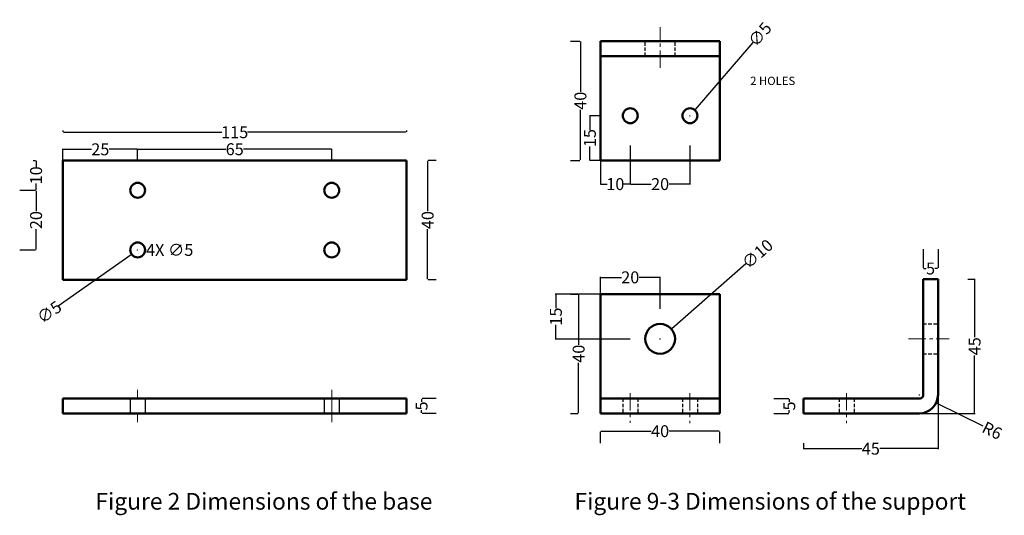
# Model space of a CAD drawing. Units: millimetres. Extents: x 1183 to 1513, y 471 to 941.
# Tile 3 of 3: x 1183 to 1513, y 775 to 941. Entities that reach past the tile are written whole.
import ezdxf

# ---------------------------------------------------------------- set-up
doc = ezdxf.new("R2010")
doc.units = ezdxf.units.MM
doc.header["$LTSCALE"] = 1.4
doc.header["$MEASUREMENT"] = 0
doc.linetypes.add('CENTER', pattern=[50.8, 31.75, -6.35, 6.35, -6.35])
doc.linetypes.add('HIDDEN', pattern=[9.525, 6.35, -3.175])
for name, color, linetype, lineweight in [('M-CNTR', 1, 'CENTER', 18), ('M-DIMS', 2, 'Continuous', 25), ('M-HIDN', 4, 'HIDDEN', 25), ('M-OUTL', 7, 'Continuous', 50), ('M-TEXT', 3, 'Continuous', 25)]:
    doc.layers.add(name, color=color, linetype=linetype, lineweight=lineweight)
doc.styles.get("Standard").update_dxf_attribs({"font": 'arial.ttf'})
doc.dimstyles.get("Standard").update_dxf_attribs({"dimtxt": 4, "dimasz": 0.18, "dimexe": 0.18, "dimexo": 10, "dimgap": 0.09, "dimtad": 0, "dimdec": 0, "dimzin": 0, "dimdsep": 46, "dimtxsty": 'Standard', "dimcen": 0.09, "dimadec": 0, "dimazin": 0, "dimtfac": 1, "dimtdec": 0, "dimtofl": 0, "dimtmove": 0, "dimatfit": 3, "dimfxl": 1, "dimtolj": 1, "dimtzin": 0, "dimarcsym": 0})

# ---------------------------------------------------------------- blocks, each defined once
blk = doc.blocks.new('*D1')
at = {"layer": 'Defpoints', "color": 0, "lineweight": 140, "ltscale": 0.13, "transparency": 16777216}
for p in [(1312.98, 903.47), (1197.98, 894.01), (1312.98, 894.01)]:
    blk.add_point(p, dxfattribs=at)
at = {"layer": 'M-DIMS', "color": 0, "lineweight": -2, "ltscale": 0.13, "transparency": 16777216}
for p, q in [((1197.98, 904.01), (1197.98, 903.65)), ((1198.16, 903.47), (1251.15, 903.47)), ((1312.8, 903.47), (1259.82, 903.47)), ((1312.98, 904.01), (1312.98, 903.65))]:
    blk.add_line(p, q, dxfattribs=at)
at = {"layer": 'M-DIMS', "color": 0, "lineweight": 140, "ltscale": 0.13, "transparency": 16777216}
for points in [[(1198.16, 903.5), (1198.16, 903.44), (1197.98, 903.47)], [(1312.8, 903.5), (1312.8, 903.44), (1312.98, 903.47)]]:
    blk.add_solid(points, dxfattribs=at)
at = {"layer": 'M-DIMS', "color": 0, "ltscale": 0.13, "transparency": 16777216, "insert": (1255.48, 903.47), "char_height": 4, "attachment_point": 5}
blk.add_mtext('\\A1;115', dxfattribs=at)
blk = doc.blocks.new('*D2')
at = {"layer": 'Defpoints', "color": 0, "lineweight": 140, "ltscale": 0.13, "transparency": 16777216}
for p in [(1287.98, 897.77), (1222.98, 884.01), (1287.98, 884.01)]:
    blk.add_point(p, dxfattribs=at)
at = {"layer": 'M-DIMS', "color": 0, "lineweight": -2, "ltscale": 0.13, "transparency": 16777216}
for p, q in [((1222.98, 894.01), (1222.98, 897.95)), ((1223.16, 897.77), (1252.5, 897.77)), ((1287.8, 897.77), (1258.46, 897.77)), ((1287.98, 894.01), (1287.98, 897.95))]:
    blk.add_line(p, q, dxfattribs=at)
at = {"layer": 'M-DIMS', "color": 0, "lineweight": 140, "ltscale": 0.13, "transparency": 16777216}
for points in [[(1223.16, 897.8), (1223.16, 897.74), (1222.98, 897.77)], [(1287.8, 897.8), (1287.8, 897.74), (1287.98, 897.77)]]:
    blk.add_solid(points, dxfattribs=at)
at = {"layer": 'M-DIMS', "color": 0, "ltscale": 0.13, "transparency": 16777216, "insert": (1255.48, 897.77), "char_height": 4, "attachment_point": 5}
blk.add_mtext('\\A1;65', dxfattribs=at)
blk = doc.blocks.new('*D3')
at = {"layer": 'Defpoints', "color": 0, "lineweight": 140, "ltscale": 0.13, "transparency": 16777216}
for p in [(1197.98, 897.74), (1197.98, 884.01), (1222.98, 884.01)]:
    blk.add_point(p, dxfattribs=at)
at = {"layer": 'M-DIMS', "color": 0, "lineweight": -2, "ltscale": 0.13, "transparency": 16777216}
for p, q in [((1197.98, 894.01), (1197.98, 897.92)), ((1198.16, 897.74), (1207.48, 897.74)), ((1222.8, 897.74), (1213.49, 897.74)), ((1222.98, 894.01), (1222.98, 897.92))]:
    blk.add_line(p, q, dxfattribs=at)
at = {"layer": 'M-DIMS', "color": 0, "lineweight": 140, "ltscale": 0.13, "transparency": 16777216}
for points in [[(1198.16, 897.77), (1198.16, 897.71), (1197.98, 897.74)], [(1222.8, 897.77), (1222.8, 897.71), (1222.98, 897.74)]]:
    blk.add_solid(points, dxfattribs=at)
at = {"layer": 'M-DIMS', "color": 0, "ltscale": 0.13, "transparency": 16777216, "insert": (1210.48, 897.74), "char_height": 4, "attachment_point": 5}
blk.add_mtext('\\A1;25', dxfattribs=at)
blk = doc.blocks.new('*D4')
at = {"layer": 'Defpoints', "color": 0, "lineweight": 140, "ltscale": 0.13, "transparency": 16777216}
for p in [(1188.97, 884.01), (1193.48, 884.01), (1193.48, 864.01)]:
    blk.add_point(p, dxfattribs=at)
at = {"layer": 'M-DIMS', "color": 0, "lineweight": -2, "ltscale": 0.13, "transparency": 16777216}
for p, q in [((1183.48, 884.01), (1188.79, 884.01)), ((1188.97, 883.83), (1188.97, 876.99)), ((1188.97, 864.19), (1188.97, 871.02)), ((1183.48, 864.01), (1188.79, 864.01))]:
    blk.add_line(p, q, dxfattribs=at)
at = {"layer": 'M-DIMS', "color": 0, "lineweight": 140, "ltscale": 0.13, "transparency": 16777216}
for points in [[(1188.94, 883.83), (1189, 883.83), (1188.97, 884.01)], [(1188.94, 864.19), (1189, 864.19), (1188.97, 864.01)]]:
    blk.add_solid(points, dxfattribs=at)
at = {"layer": 'M-DIMS', "color": 0, "ltscale": 0.13, "transparency": 16777216, "insert": (1188.97, 874.01), "char_height": 4, "attachment_point": 5, "rotation": 90}
blk.add_mtext('\\A1;20', dxfattribs=at)
blk = doc.blocks.new('*D5')
at = {"layer": 'Defpoints', "color": 0, "lineweight": 140, "ltscale": 0.13, "transparency": 16777216}
for p in [(1197.98, 894.01), (1188.97, 884.01), (1197.98, 884.01)]:
    blk.add_point(p, dxfattribs=at)
at = {"layer": 'M-DIMS', "color": 0, "lineweight": -2, "ltscale": 0.13, "transparency": 16777216}
for p, q in [((1187.98, 894.01), (1188.79, 894.01)), ((1188.97, 893.83), (1188.97, 891.77)), ((1187.98, 884.01), (1188.79, 884.01)), ((1188.97, 884.19), (1188.97, 886.25))]:
    blk.add_line(p, q, dxfattribs=at)
at = {"layer": 'M-DIMS', "color": 0, "lineweight": 140, "ltscale": 0.13, "transparency": 16777216}
for points in [[(1188.94, 893.83), (1189, 893.83), (1188.97, 894.01)], [(1188.94, 884.19), (1189, 884.19), (1188.97, 884.01)]]:
    blk.add_solid(points, dxfattribs=at)
at = {"layer": 'M-DIMS', "color": 0, "ltscale": 0.13, "transparency": 16777216, "insert": (1188.97, 889.01), "char_height": 4, "attachment_point": 5, "rotation": 90}
blk.add_mtext('\\A1;10', dxfattribs=at)
blk = doc.blocks.new('*D6')
at = {"layer": 'Defpoints', "color": 0, "lineweight": 140, "ltscale": 0.13, "transparency": 16777216}
for p in [(1225.03, 865.44), (1220.94, 862.57)]:
    blk.add_point(p, dxfattribs=at)
at = {"layer": 'M-DIMS', "color": 0, "lineweight": -2, "ltscale": 0.13, "transparency": 16777216}
for p, q in [((1222.89, 864.01), (1223.07, 864.01)), ((1222.98, 863.92), (1222.98, 864.1)), ((1196.32, 845.25), (1220.79, 862.46))]:
    blk.add_line(p, q, dxfattribs=at)
at = {"layer": 'M-DIMS', "color": 0, "lineweight": 140, "ltscale": 0.13, "transparency": 16777216}
blk.add_solid([(1220.77, 862.49), (1220.81, 862.44), (1220.94, 862.57)], dxfattribs=at)
at = {"layer": 'M-DIMS', "color": 0, "ltscale": 0.13, "transparency": 16777216, "insert": (1193.38, 843.18), "char_height": 4, "attachment_point": 5, "rotation": 35.1278}
blk.add_mtext('\\A1;∅5', dxfattribs=at)
blk = doc.blocks.new('*D7')
at = {"layer": 'Defpoints', "color": 0, "lineweight": 140, "ltscale": 0.13, "transparency": 16777216}
for p in [(1312.98, 894.01), (1312.98, 854.01), (1320.09, 854.01)]:
    blk.add_point(p, dxfattribs=at)
at = {"layer": 'M-DIMS', "color": 0, "lineweight": -2, "ltscale": 0.13, "transparency": 16777216}
for p, q in [((1320.09, 893.83), (1320.09, 877.03)), ((1322.98, 894.01), (1320.27, 894.01)), ((1320.09, 854.19), (1320.09, 870.98)), ((1322.98, 854.01), (1320.27, 854.01))]:
    blk.add_line(p, q, dxfattribs=at)
at = {"layer": 'M-DIMS', "color": 0, "lineweight": 140, "ltscale": 0.13, "transparency": 16777216}
for points in [[(1320.06, 893.83), (1320.12, 893.83), (1320.09, 894.01)], [(1320.06, 854.19), (1320.12, 854.19), (1320.09, 854.01)]]:
    blk.add_solid(points, dxfattribs=at)
at = {"layer": 'M-DIMS', "color": 0, "ltscale": 0.13, "transparency": 16777216, "insert": (1320.09, 874.01), "char_height": 4, "attachment_point": 5, "rotation": 90}
blk.add_mtext('\\A1;40', dxfattribs=at)
blk = doc.blocks.new('*D8')
at = {"layer": 'Defpoints', "color": 0, "lineweight": 140, "ltscale": 0.13, "transparency": 16777216}
for p in [(1371.24, 934.01), (1377.94, 934.01), (1377.94, 894.01)]:
    blk.add_point(p, dxfattribs=at)
at = {"layer": 'M-DIMS', "color": 0, "lineweight": -2, "ltscale": 0.13, "transparency": 16777216}
for p, q in [((1367.94, 934.01), (1371.06, 934.01)), ((1371.24, 933.83), (1371.24, 917.03)), ((1371.24, 894.19), (1371.24, 910.98)), ((1367.94, 894.01), (1371.06, 894.01))]:
    blk.add_line(p, q, dxfattribs=at)
at = {"layer": 'M-DIMS', "color": 0, "lineweight": 140, "ltscale": 0.13, "transparency": 16777216}
for points in [[(1371.21, 933.83), (1371.27, 933.83), (1371.24, 934.01)], [(1371.21, 894.19), (1371.27, 894.19), (1371.24, 894.01)]]:
    blk.add_solid(points, dxfattribs=at)
at = {"layer": 'M-DIMS', "color": 0, "ltscale": 0.13, "transparency": 16777216, "insert": (1371.24, 914.01), "char_height": 4, "attachment_point": 5, "rotation": 90}
blk.add_mtext('\\A1;40', dxfattribs=at)
blk = doc.blocks.new('*D9')
at = {"layer": 'Defpoints', "color": 0, "lineweight": 140, "ltscale": 0.13, "transparency": 16777216}
for p in [(1377.94, 909.01), (1387.94, 909.01), (1377.94, 886.08)]:
    blk.add_point(p, dxfattribs=at)
at = {"layer": 'M-DIMS', "color": 0, "lineweight": -2, "ltscale": 0.13, "transparency": 16777216}
for p, q in [((1377.94, 899.01), (1377.94, 885.9)), ((1387.94, 899.01), (1387.94, 885.9)), ((1378.12, 886.08), (1380.18, 886.08)), ((1387.76, 886.08), (1385.7, 886.08))]:
    blk.add_line(p, q, dxfattribs=at)
at = {"layer": 'M-DIMS', "color": 0, "lineweight": 140, "ltscale": 0.13, "transparency": 16777216}
for points in [[(1378.12, 886.11), (1378.12, 886.05), (1377.94, 886.08)], [(1387.76, 886.11), (1387.76, 886.05), (1387.94, 886.08)]]:
    blk.add_solid(points, dxfattribs=at)
at = {"layer": 'M-DIMS', "color": 0, "ltscale": 0.13, "transparency": 16777216, "insert": (1382.94, 886.08), "char_height": 4, "attachment_point": 5}
blk.add_mtext('\\A1;10', dxfattribs=at)
blk = doc.blocks.new('*D10')
at = {"layer": 'Defpoints', "color": 0, "lineweight": 140, "ltscale": 0.13, "transparency": 16777216}
for p in [(1387.94, 909.01), (1407.94, 909.01), (1407.94, 886.08)]:
    blk.add_point(p, dxfattribs=at)
at = {"layer": 'M-DIMS', "color": 0, "lineweight": -2, "ltscale": 0.13, "transparency": 16777216}
for p, q in [((1387.94, 899.01), (1387.94, 885.9)), ((1407.94, 899.01), (1407.94, 885.9)), ((1388.12, 886.08), (1394.96, 886.08)), ((1407.76, 886.08), (1400.92, 886.08))]:
    blk.add_line(p, q, dxfattribs=at)
at = {"layer": 'M-DIMS', "color": 0, "lineweight": 140, "ltscale": 0.13, "transparency": 16777216}
for points in [[(1388.12, 886.11), (1388.12, 886.05), (1387.94, 886.08)], [(1407.76, 886.11), (1407.76, 886.05), (1407.94, 886.08)]]:
    blk.add_solid(points, dxfattribs=at)
at = {"layer": 'M-DIMS', "color": 0, "ltscale": 0.13, "transparency": 16777216, "insert": (1397.94, 886.08), "char_height": 4, "attachment_point": 5}
blk.add_mtext('\\A1;20', dxfattribs=at)
blk = doc.blocks.new('*D11')
at = {"layer": 'Defpoints', "color": 0, "lineweight": 140, "ltscale": 0.13, "transparency": 16777216}
for p in [(1374.42, 909.01), (1387.94, 909.01), (1387.94, 894.01)]:
    blk.add_point(p, dxfattribs=at)
at = {"layer": 'M-DIMS', "color": 0, "lineweight": -2, "ltscale": 0.13, "transparency": 16777216}
for p, q in [((1377.94, 909.01), (1374.24, 909.01)), ((1374.42, 908.83), (1374.42, 904.29)), ((1374.42, 894.19), (1374.42, 898.72)), ((1377.94, 894.01), (1374.24, 894.01))]:
    blk.add_line(p, q, dxfattribs=at)
at = {"layer": 'M-DIMS', "color": 0, "lineweight": 140, "ltscale": 0.13, "transparency": 16777216}
for points in [[(1374.39, 908.83), (1374.45, 908.83), (1374.42, 909.01)], [(1374.39, 894.19), (1374.45, 894.19), (1374.42, 894.01)]]:
    blk.add_solid(points, dxfattribs=at)
at = {"layer": 'M-DIMS', "color": 0, "ltscale": 0.13, "transparency": 16777216, "insert": (1374.42, 901.51), "char_height": 4, "attachment_point": 5, "rotation": 90}
blk.add_mtext('\\A1;15', dxfattribs=at)
blk = doc.blocks.new('*D12')
at = {"layer": 'Defpoints', "color": 0, "lineweight": 140, "ltscale": 0.13, "transparency": 16777216}
for p in [(1409.57, 910.9), (1406.31, 907.11)]:
    blk.add_point(p, dxfattribs=at)
at = {"layer": 'M-DIMS', "color": 0, "lineweight": -2, "ltscale": 0.13, "transparency": 16777216}
for p, q in [((1429.01, 933.53), (1409.68, 911.04)), ((1407.85, 909.01), (1408.03, 909.01)), ((1407.94, 908.92), (1407.94, 909.1))]:
    blk.add_line(p, q, dxfattribs=at)
at = {"layer": 'M-DIMS', "color": 0, "lineweight": 140, "ltscale": 0.13, "transparency": 16777216}
blk.add_solid([(1409.66, 911.06), (1409.71, 911.02), (1409.57, 910.9)], dxfattribs=at)
at = {"layer": 'M-DIMS', "color": 0, "ltscale": 0.13, "transparency": 16777216, "insert": (1431.35, 936.26), "char_height": 4, "attachment_point": 5, "rotation": 49.3316}
blk.add_mtext('\\A1;∅5', dxfattribs=at)
blk = doc.blocks.new('*D13')
at = {"layer": 'Defpoints', "color": 0, "lineweight": 140, "ltscale": 0.13, "transparency": 16777216}
for p in [(1312.98, 814.23), (1318.05, 814.23), (1312.98, 809.23)]:
    blk.add_point(p, dxfattribs=at)
at = {"layer": 'M-DIMS', "color": 0, "lineweight": -2, "ltscale": 0.13, "transparency": 16777216}
for p, q in [((1318.05, 814.05), (1318.05, 813.14)), ((1322.98, 814.23), (1318.23, 814.23)), ((1318.05, 809.41), (1318.05, 810.31)), ((1322.98, 809.23), (1318.23, 809.23))]:
    blk.add_line(p, q, dxfattribs=at)
at = {"layer": 'M-DIMS', "color": 0, "lineweight": 140, "ltscale": 0.13, "transparency": 16777216}
for points in [[(1318.02, 814.05), (1318.08, 814.05), (1318.05, 814.23)], [(1318.02, 809.41), (1318.08, 809.41), (1318.05, 809.23)]]:
    blk.add_solid(points, dxfattribs=at)
at = {"layer": 'M-DIMS', "color": 0, "ltscale": 0.13, "transparency": 16777216, "insert": (1318.05, 811.73), "char_height": 4, "attachment_point": 5, "rotation": 90}
blk.add_mtext('\\A1;5', dxfattribs=at)
blk = doc.blocks.new('*D14')
at = {"layer": 'Defpoints', "color": 0, "lineweight": 140, "ltscale": 0.13, "transparency": 16777216}
for p in [(1377.94, 854.83), (1377.94, 834.23), (1397.94, 834.23)]:
    blk.add_point(p, dxfattribs=at)
at = {"layer": 'M-DIMS', "color": 0, "lineweight": -2, "ltscale": 0.13, "transparency": 16777216}
for p, q in [((1377.94, 844.23), (1377.94, 855.01)), ((1378.12, 854.83), (1384.96, 854.83)), ((1397.76, 854.83), (1390.92, 854.83)), ((1397.94, 844.23), (1397.94, 855.01))]:
    blk.add_line(p, q, dxfattribs=at)
at = {"layer": 'M-DIMS', "color": 0, "lineweight": 140, "ltscale": 0.13, "transparency": 16777216}
for points in [[(1378.12, 854.86), (1378.12, 854.8), (1377.94, 854.83)], [(1397.76, 854.86), (1397.76, 854.8), (1397.94, 854.83)]]:
    blk.add_solid(points, dxfattribs=at)
at = {"layer": 'M-DIMS', "color": 0, "ltscale": 0.13, "transparency": 16777216, "insert": (1387.94, 854.83), "char_height": 4, "attachment_point": 5}
blk.add_mtext('\\A1;20', dxfattribs=at)
blk = doc.blocks.new('*D15')
at = {"layer": 'Defpoints', "color": 0, "lineweight": 140, "ltscale": 0.13, "transparency": 16777216}
for p in [(1370.65, 849.23), (1377.94, 849.23), (1377.94, 809.23)]:
    blk.add_point(p, dxfattribs=at)
at = {"layer": 'M-DIMS', "color": 0, "lineweight": -2, "ltscale": 0.13, "transparency": 16777216}
for p, q in [((1367.94, 849.23), (1370.47, 849.23)), ((1370.65, 849.05), (1370.65, 832.25)), ((1370.65, 809.41), (1370.65, 826.2)), ((1367.94, 809.23), (1370.47, 809.23))]:
    blk.add_line(p, q, dxfattribs=at)
at = {"layer": 'M-DIMS', "color": 0, "lineweight": 140, "ltscale": 0.13, "transparency": 16777216}
for points in [[(1370.62, 849.05), (1370.68, 849.05), (1370.65, 849.23)], [(1370.62, 809.41), (1370.68, 809.41), (1370.65, 809.23)]]:
    blk.add_solid(points, dxfattribs=at)
at = {"layer": 'M-DIMS', "color": 0, "ltscale": 0.13, "transparency": 16777216, "insert": (1370.65, 829.23), "char_height": 4, "attachment_point": 5, "rotation": 90}
blk.add_mtext('\\A1;40', dxfattribs=at)
blk = doc.blocks.new('*D16')
at = {"layer": 'Defpoints', "color": 0, "lineweight": 140, "ltscale": 0.13, "transparency": 16777216}
for p in [(1377.94, 809.23), (1417.94, 809.23), (1417.94, 803.28)]:
    blk.add_point(p, dxfattribs=at)
at = {"layer": 'M-DIMS', "color": 0, "lineweight": -2, "ltscale": 0.13, "transparency": 16777216}
for p, q in [((1377.94, 799.23), (1377.94, 803.1)), ((1378.12, 803.28), (1394.91, 803.28)), ((1417.76, 803.28), (1400.97, 803.28)), ((1417.94, 799.23), (1417.94, 803.1))]:
    blk.add_line(p, q, dxfattribs=at)
at = {"layer": 'M-DIMS', "color": 0, "lineweight": 140, "ltscale": 0.13, "transparency": 16777216}
for points in [[(1378.12, 803.31), (1378.12, 803.25), (1377.94, 803.28)], [(1417.76, 803.31), (1417.76, 803.25), (1417.94, 803.28)]]:
    blk.add_solid(points, dxfattribs=at)
at = {"layer": 'M-DIMS', "color": 0, "ltscale": 0.13, "transparency": 16777216, "insert": (1397.94, 803.28), "char_height": 4, "attachment_point": 5}
blk.add_mtext('\\A1;40', dxfattribs=at)
blk = doc.blocks.new('*D17')
at = {"layer": 'Defpoints', "color": 0, "lineweight": 140, "ltscale": 0.13, "transparency": 16777216}
for p in [(1401.7, 837.52), (1394.17, 830.94)]:
    blk.add_point(p, dxfattribs=at)
at = {"layer": 'M-DIMS', "color": 0, "lineweight": -2, "ltscale": 0.13, "transparency": 16777216}
for p, q in [((1426.66, 859.33), (1401.84, 837.63)), ((1397.85, 834.23), (1398.03, 834.23)), ((1397.94, 834.14), (1397.94, 834.32))]:
    blk.add_line(p, q, dxfattribs=at)
at = {"layer": 'M-DIMS', "color": 0, "lineweight": 140, "ltscale": 0.13, "transparency": 16777216}
blk.add_solid([(1401.82, 837.66), (1401.86, 837.61), (1401.7, 837.52)], dxfattribs=at)
at = {"layer": 'M-DIMS', "color": 0, "ltscale": 0.13, "transparency": 16777216, "insert": (1430.52, 862.7), "char_height": 4, "attachment_point": 5, "rotation": 41.1476}
blk.add_mtext('\\A1;∅10', dxfattribs=at)
blk = doc.blocks.new('*D18')
at = {"layer": 'Defpoints', "color": 0, "lineweight": 140, "ltscale": 0.13, "transparency": 16777216}
for p in [(1484.75, 815.48), (1490.36, 812.72)]:
    blk.add_point(p, dxfattribs=at)
at = {"layer": 'M-DIMS', "color": 0, "lineweight": -2, "ltscale": 0.13, "transparency": 16777216}
for p, q in [((1484.66, 815.48), (1484.84, 815.48)), ((1484.75, 815.39), (1484.75, 815.57)), ((1506.15, 804.95), (1490.52, 812.64))]:
    blk.add_line(p, q, dxfattribs=at)
at = {"layer": 'M-DIMS', "color": 0, "lineweight": 140, "ltscale": 0.13, "transparency": 16777216}
blk.add_solid([(1490.53, 812.66), (1490.5, 812.61), (1490.36, 812.72)], dxfattribs=at)
at = {"layer": 'M-DIMS', "color": 0, "ltscale": 0.13, "transparency": 16777216, "insert": (1509.13, 803.48), "char_height": 4, "attachment_point": 5, "rotation": 333.8095}
blk.add_mtext('\\A1;R6', dxfattribs=at)
blk = doc.blocks.new('*D19')
at = {"layer": 'Defpoints', "color": 0, "lineweight": 140, "ltscale": 0.13, "transparency": 16777216}
for p in [(1363.03, 849.23), (1397.94, 849.23), (1397.94, 834.14)]:
    blk.add_point(p, dxfattribs=at)
at = {"layer": 'M-DIMS', "color": 0, "lineweight": -2, "ltscale": 0.13, "transparency": 16777216}
for p, q in [((1387.94, 849.23), (1362.85, 849.23)), ((1363.03, 849.05), (1363.03, 844.46)), ((1363.03, 834.32), (1363.03, 838.9)), ((1387.94, 834.14), (1362.85, 834.14))]:
    blk.add_line(p, q, dxfattribs=at)
at = {"layer": 'M-DIMS', "color": 0, "lineweight": 140, "ltscale": 0.13, "transparency": 16777216}
for points in [[(1363, 849.05), (1363.06, 849.05), (1363.03, 849.23)], [(1363, 834.32), (1363.06, 834.32), (1363.03, 834.14)]]:
    blk.add_solid(points, dxfattribs=at)
at = {"layer": 'M-DIMS', "color": 0, "ltscale": 0.13, "transparency": 16777216, "insert": (1363.03, 841.68), "char_height": 4, "attachment_point": 5, "rotation": 90}
blk.add_mtext('\\A1;15', dxfattribs=at)
blk = doc.blocks.new('*D20')
at = {"layer": 'Defpoints', "color": 0, "lineweight": 140, "ltscale": 0.13, "transparency": 16777216}
for p in [(1491, 857.79), (1486, 854.23), (1491, 854.23)]:
    blk.add_point(p, dxfattribs=at)
at = {"layer": 'M-DIMS', "color": 0, "lineweight": -2, "ltscale": 0.13, "transparency": 16777216}
for p, q in [((1486, 864.23), (1486, 857.97)), ((1491, 864.23), (1491, 857.97)), ((1486.18, 857.79), (1487.08, 857.79)), ((1490.82, 857.79), (1489.91, 857.79))]:
    blk.add_line(p, q, dxfattribs=at)
at = {"layer": 'M-DIMS', "color": 0, "lineweight": 140, "ltscale": 0.13, "transparency": 16777216}
for points in [[(1486.18, 857.82), (1486.18, 857.76), (1486, 857.79)], [(1490.82, 857.82), (1490.82, 857.76), (1491, 857.79)]]:
    blk.add_solid(points, dxfattribs=at)
at = {"layer": 'M-DIMS', "color": 0, "ltscale": 0.13, "transparency": 16777216, "insert": (1488.5, 857.79), "char_height": 4, "attachment_point": 5}
blk.add_mtext('\\A1;5', dxfattribs=at)
blk = doc.blocks.new('*D21')
at = {"layer": 'Defpoints', "color": 0, "lineweight": 140, "ltscale": 0.13, "transparency": 16777216}
for p in [(1441.17, 814.23), (1446, 814.23), (1446, 809.23)]:
    blk.add_point(p, dxfattribs=at)
at = {"layer": 'M-DIMS', "color": 0, "lineweight": -2, "ltscale": 0.13, "transparency": 16777216}
for p, q in [((1436, 814.23), (1440.99, 814.23)), ((1441.17, 814.05), (1441.17, 813.14)), ((1436, 809.23), (1440.99, 809.23)), ((1441.17, 809.41), (1441.17, 810.31))]:
    blk.add_line(p, q, dxfattribs=at)
at = {"layer": 'M-DIMS', "color": 0, "lineweight": 140, "ltscale": 0.13, "transparency": 16777216}
for points in [[(1441.14, 814.05), (1441.2, 814.05), (1441.17, 814.23)], [(1441.14, 809.41), (1441.2, 809.41), (1441.17, 809.23)]]:
    blk.add_solid(points, dxfattribs=at)
at = {"layer": 'M-DIMS', "color": 0, "ltscale": 0.13, "transparency": 16777216, "insert": (1441.17, 811.73), "char_height": 4, "attachment_point": 5, "rotation": 90}
blk.add_mtext('\\A1;5', dxfattribs=at)
blk = doc.blocks.new('*D46')
at = {"layer": 'Defpoints', "color": 0, "lineweight": 140, "ltscale": 1.4, "transparency": 16777216}
for p in [(1491, 854.23), (1446, 809.23), (1491, 797.42)]:
    blk.add_point(p, dxfattribs=at)
at = {"layer": 'M-DIMS', "color": 0, "lineweight": -2, "ltscale": 1.4, "transparency": 16777216}
for p, q in [((1491, 844.23), (1491, 797.24)), ((1446, 799.23), (1446, 797.24)), ((1446.18, 797.42), (1465.45, 797.42)), ((1490.82, 797.42), (1471.55, 797.42))]:
    blk.add_line(p, q, dxfattribs=at)
at = {"layer": 'M-DIMS', "color": 0, "lineweight": 140, "ltscale": 1.4, "transparency": 16777216}
for points in [[(1446.18, 797.45), (1446.18, 797.39), (1446, 797.42)], [(1490.82, 797.45), (1490.82, 797.39), (1491, 797.42)]]:
    blk.add_solid(points, dxfattribs=at)
at = {"layer": 'M-DIMS', "color": 0, "ltscale": 1.4, "transparency": 16777216, "insert": (1468.5, 797.42), "char_height": 4, "attachment_point": 5}
blk.add_mtext('\\A1;45', dxfattribs=at)
blk = doc.blocks.new('*D47')
at = {"layer": 'Defpoints', "color": 0, "lineweight": 140, "ltscale": 1.4, "transparency": 16777216}
for p in [(1491, 854.23), (1503.24, 854.23), (1446, 809.23)]:
    blk.add_point(p, dxfattribs=at)
at = {"layer": 'M-DIMS', "color": 0, "lineweight": -2, "ltscale": 1.4, "transparency": 16777216}
for p, q in [((1501, 854.23), (1503.42, 854.23)), ((1503.24, 854.05), (1503.24, 834.78)), ((1503.24, 809.41), (1503.24, 828.68)), ((1456, 809.23), (1503.42, 809.23))]:
    blk.add_line(p, q, dxfattribs=at)
at = {"layer": 'M-DIMS', "color": 0, "lineweight": 140, "ltscale": 1.4, "transparency": 16777216}
for points in [[(1503.21, 854.05), (1503.27, 854.05), (1503.24, 854.23)], [(1503.21, 809.41), (1503.27, 809.41), (1503.24, 809.23)]]:
    blk.add_solid(points, dxfattribs=at)
at = {"layer": 'M-DIMS', "color": 0, "ltscale": 1.4, "transparency": 16777216, "insert": (1503.24, 831.73), "char_height": 4, "attachment_point": 5, "rotation": 90}
blk.add_mtext('\\A1;45', dxfattribs=at)
blk = doc.blocks.new('*D55')
at = {"layer": 'Defpoints', "color": 0, "lineweight": 140, "ltscale": 1.4, "transparency": 16777216}
for p in [(1220.48, 864), (1225.48, 864.01)]:
    blk.add_point(p, dxfattribs=at)
at = {"layer": 'M-DIMS', "color": 0, "lineweight": -2, "ltscale": 1.4, "transparency": 16777216}
for p, q in [((1222.89, 864.01), (1223.07, 864.01)), ((1222.98, 863.92), (1222.98, 864.1)), ((1225.84, 864.01), (1225.66, 864.01))]:
    blk.add_line(p, q, dxfattribs=at)
at = {"layer": 'M-DIMS', "color": 0, "lineweight": 140, "ltscale": 1.4, "transparency": 16777216}
blk.add_solid([(1225.66, 864.04), (1225.66, 863.98), (1225.48, 864.01)], dxfattribs=at)
at = {"layer": 'M-DIMS', "color": 0, "ltscale": 1.4, "transparency": 16777216, "insert": (1233.71, 864.02), "char_height": 4, "attachment_point": 5, "rotation": 0.0833}
blk.add_mtext('\\A1;4X ∅5', dxfattribs=at)

msp = doc.modelspace()

# ---------------------------------------------------------------- linework, layer by layer
at = {"layer": 'M-CNTR', "ltscale": 0.13}
for p, q in [((1397.9372, 925.1022), (1397.9372, 938.707)), ((1481.1697, 834.2258), (1494.6893, 834.2258)), ((1387.9372, 816.0346), (1387.9372, 806.0807)), ((1407.9372, 816.0346), (1407.9372, 805.9701)), ((1460.3802, 816.0346), (1460.3802, 805.9701))]:
    msp.add_line(p, q, dxfattribs=at)
at = {"layer": 'M-CNTR'}
for p, q in [((1222.9815, 814.2258), (1222.9815, 817.1552)), ((1287.9815, 814.2258), (1287.9815, 817.1552)), ((1222.9815, 809.2258), (1222.9815, 806.2964)), ((1287.9815, 809.2258), (1287.9815, 806.2964))]:
    msp.add_line(p, q, dxfattribs=at)
at = {"layer": 'M-CNTR', "ltscale": 2}
msp.add_line((1287.9815, 814.2258), (1287.9815, 809.2258), dxfattribs=at)
at = {"layer": 'M-HIDN', "ltscale": 0.13}
for p, q in [((1392.9372, 929.0064), (1392.9372, 934.0064)), ((1402.9372, 929.0064), (1402.9372, 934.0064)), ((1485.9973, 839.2258), (1490.9973, 839.2258)), ((1485.9973, 829.2258), (1490.9973, 829.2258)), ((1385.4372, 814.2258), (1385.4372, 809.2258)), ((1390.4372, 814.2258), (1390.4372, 809.2258)), ((1405.4372, 814.2258), (1405.4372, 809.2258)), ((1410.4372, 814.2258), (1410.4372, 809.2258)), ((1457.8802, 814.2258), (1457.8802, 809.2258)), ((1462.8802, 814.2258), (1462.8802, 809.2258))]:
    msp.add_line(p, q, dxfattribs=at)
at = {"layer": 'M-HIDN', "ltscale": 2}
for p, q in [((1220.4815, 814.2258), (1220.4815, 809.2258)), ((1225.4815, 814.2258), (1225.4815, 809.2258)), ((1285.4815, 814.2258), (1285.4815, 809.2258)), ((1290.4815, 814.2258), (1290.4815, 809.2258))]:
    msp.add_line(p, q, dxfattribs=at)
at = {"layer": 'M-OUTL', "ltscale": 0.13}
for p, q in [((1377.9372, 934.0064), (1417.9372, 934.0064)), ((1377.9372, 894.0064), (1377.9372, 934.0064)), ((1417.9372, 934.0064), (1417.9372, 894.0064)), ((1377.9372, 929.0064), (1417.9372, 929.0064)), ((1417.9372, 894.0064), (1377.9372, 894.0064)), ((1485.9973, 815.2258), (1485.9973, 854.2258)), ((1485.9973, 854.2258), (1490.9973, 854.2258)), ((1490.9973, 815.4758), (1490.9973, 854.2258)), ((1377.9372, 849.2258), (1417.9372, 849.2258)), ((1377.9372, 809.2258), (1377.9372, 849.2258)), ((1417.9372, 849.2258), (1417.9372, 809.2258)), ((1417.9372, 814.2258), (1377.9372, 814.2258)), ((1445.9973, 814.2258), (1445.9973, 809.2258)), ((1445.9973, 814.2258), (1484.9973, 814.2258)), ((1417.9372, 809.2258), (1377.9372, 809.2258)), ((1445.9973, 809.2258), (1484.7473, 809.2258))]:
    msp.add_line(p, q, dxfattribs=at)
at = {"layer": 'M-OUTL'}
for p, q in [((1197.9815, 894.0064), (1312.9815, 894.0064)), ((1197.9815, 894.0064), (1197.9815, 854.0064)), ((1312.9815, 854.0064), (1312.9815, 894.0064)), ((1197.9815, 854.0064), (1312.9815, 854.0064)), ((1197.9815, 814.2258), (1197.9815, 809.2258)), ((1197.9815, 814.2258), (1312.9815, 814.2258)), ((1312.9815, 814.2258), (1312.9815, 809.2258)), ((1312.9815, 809.2258), (1197.9815, 809.2258))]:
    msp.add_line(p, q, dxfattribs=at)
at = {"layer": 'M-OUTL', "ltscale": 0.13}
for centre, radius in [((1387.9372, 909.0064), 2.5), ((1407.9372, 909.0064), 2.5), ((1397.9372, 834.2258), 5)]:
    msp.add_circle(centre, radius, dxfattribs=at)
at = {"layer": 'M-OUTL'}
for centre in [(1222.9815, 884.0064), (1287.9815, 884.0064), (1222.9815, 864.0064), (1287.9815, 864.0064)]:
    msp.add_circle(centre, 2.5, dxfattribs=at)
at = {"layer": 'M-OUTL', "ltscale": 0.13}
for centre, radius in [((1484.7473, 815.4758), 6.25), ((1484.9973, 815.2258), 1)]:
    msp.add_arc(centre, radius, 270, 0, dxfattribs=at)

# ---------------------------------------------------------------- texts
at = {"layer": 'M-TEXT', "ltscale": 0.13}
for s, height, p in [('2 HOLES', 2.77686, (1428.1095, 919.2891)), ('Figure 2 Dimensions of the base ', 5.601941, (1208.8339, 776.9865)), ('Figure 9-3 Dimensions of the support ', 5.601941, (1369.2621, 776.9865))]:
    msp.add_text(s, height=height, dxfattribs=at).set_placement(p)

# ---------------------------------------------------------------- dimensions: what is measured, and where the dimension line sits
at = {"layer": 'M-DIMS', "ltscale": 0.13}
for p1, p2, picture, middle in [((1406.308, 907.1101), (1409.5664, 910.9026), '*D12', (1431.3517, 936.2585)), ((1394.1722, 830.9358), (1401.7023, 837.5158), '*D17', (1430.5216, 862.6987)), ((1225.0262, 865.4449), (1220.9368, 862.5679), '*D6', (1193.3774, 843.1788))]:
    dim = msp.add_diameter_dim_2p(p1=p1, p2=p2, dimstyle='Standard', override={"dimclrd": 0, "dimclre": 0, "dimclrt": 0}, dxfattribs=at)
    dim.commit()
    dim.dimension.update_dxf_attribs({"geometry": picture, "text_midpoint": middle, "dimtype": 163})
for base, p1, p2, picture, middle in [((1371.2376, 934.0064), (1377.9372, 894.0064), (1377.9372, 934.0064), '*D8', (1371.2376, 914.0064)), ((1374.4218, 909.0064), (1387.9372, 894.0064), (1387.9372, 909.0064), '*D11', (1374.4218, 901.5064)), ((1188.9695, 884.0064), (1197.9815, 894.0064), (1197.9815, 884.0064), '*D5', (1188.9695, 889.0064)), ((1320.0875, 854.0064), (1312.9815, 894.0064), (1312.9815, 854.0064), '*D7', (1320.0875, 874.0064)), ((1188.9695, 884.0064), (1193.4815, 864.0064), (1193.4815, 884.0064), '*D4', (1188.9695, 874.0064)), ((1363.0328, 849.2258), (1397.9372, 834.1358), (1397.9372, 849.2258), '*D19', (1363.0328, 841.6808)), ((1370.6485, 849.2258), (1377.9372, 809.2258), (1377.9372, 849.2258), '*D15', (1370.6485, 829.2258)), ((1318.0513, 814.2258), (1312.9815, 809.2258), (1312.9815, 814.2258), '*D13', (1318.0513, 811.7258)), ((1441.1718, 814.2258), (1445.9973, 809.2258), (1445.9973, 814.2258), '*D21', (1441.1718, 811.7258))]:
    dim = msp.add_linear_dim(base=base, p1=p1, p2=p2, angle=90, dimstyle='Standard', override={"dimclrd": 0, "dimclre": 0, "dimclrt": 0}, dxfattribs=at)
    dim.commit()
    dim.dimension.update_dxf_attribs({"geometry": picture, "text_midpoint": middle})
for base, p1, p2, picture, middle in [((1377.9372, 886.0819), (1387.9372, 909.0064), (1377.9372, 909.0064), '*D9', (1382.9372, 886.0819)), ((1407.9372, 886.0819), (1387.9372, 909.0064), (1407.9372, 909.0064), '*D10', (1397.9372, 886.0819)), ((1312.9815, 903.466), (1197.9815, 894.0064), (1312.9815, 894.0064), '*D1', (1255.4815, 903.466)), ((1197.9815, 897.7352), (1222.9815, 884.0064), (1197.9815, 884.0064), '*D3', (1210.4815, 897.7352)), ((1287.9815, 897.7652), (1222.9815, 884.0064), (1287.9815, 884.0064), '*D2', (1255.4815, 897.7652)), ((1490.9973, 857.7915), (1485.9973, 854.2258), (1490.9973, 854.2258), '*D20', (1488.4973, 857.7915)), ((1377.9372, 854.8303), (1397.9372, 834.2258), (1377.9372, 834.2258), '*D14', (1387.9372, 854.8303)), ((1417.9372, 803.2829), (1377.9372, 809.2258), (1417.9372, 809.2258), '*D16', (1397.9372, 803.2829))]:
    dim = msp.add_linear_dim(base=base, p1=p1, p2=p2, dimstyle='Standard', override={"dimclrd": 0, "dimclre": 0, "dimclrt": 0}, dxfattribs=at)
    dim.commit()
    dim.dimension.update_dxf_attribs({"geometry": picture, "text_midpoint": middle})
at = {"layer": 'M-DIMS', "ltscale": 1.4}
dim = msp.add_diameter_dim_2p(p1=(1220.4815, 864.0027), p2=(1225.4815, 864.01), text='4X <>', dimstyle='Standard', override={"dimdec": 0, "dimlfac": 1, "dimrnd": 0, "dimzin": 0, "dimdsep": 46, "dimlunit": 2}, dxfattribs=at)
dim.commit()
dim.dimension.update_dxf_attribs({"geometry": '*D55', "text_midpoint": (1233.705, 864.022)})
dim = msp.add_linear_dim(base=(1490.9973, 797.4201), p1=(1445.9973, 809.2258), p2=(1490.9973, 854.2258), dimstyle='Standard', override={"dimdec": 0, "dimlfac": 1, "dimrnd": 0, "dimzin": 0, "dimdsep": 46, "dimlunit": 2}, dxfattribs=at)
dim.commit()
dim.dimension.update_dxf_attribs({"geometry": '*D46', "text_midpoint": (1468.4973, 797.4201)})
dim = msp.add_linear_dim(base=(1503.2393, 854.2258), p1=(1445.9973, 809.2258), p2=(1490.9973, 854.2258), angle=90, dimstyle='Standard', override={"dimdec": 0, "dimlfac": 1, "dimrnd": 0, "dimzin": 0, "dimdsep": 46, "dimlunit": 2}, dxfattribs=at)
dim.commit()
dim.dimension.update_dxf_attribs({"geometry": '*D47', "text_midpoint": (1503.2393, 831.7258)})
at = {"layer": 'M-DIMS', "ltscale": 0.13}
dim = msp.add_radius_dim(center=(1484.7473, 815.4758), mpoint=(1490.3556, 812.7173), dimstyle='Standard', override={"dimclrd": 0, "dimclre": 0, "dimclrt": 0}, dxfattribs=at)
dim.commit()
dim.dimension.update_dxf_attribs({"geometry": '*D18', "text_midpoint": (1509.1272, 803.4844), "dimtype": 164})

doc.saveas('drawing.dxf')
